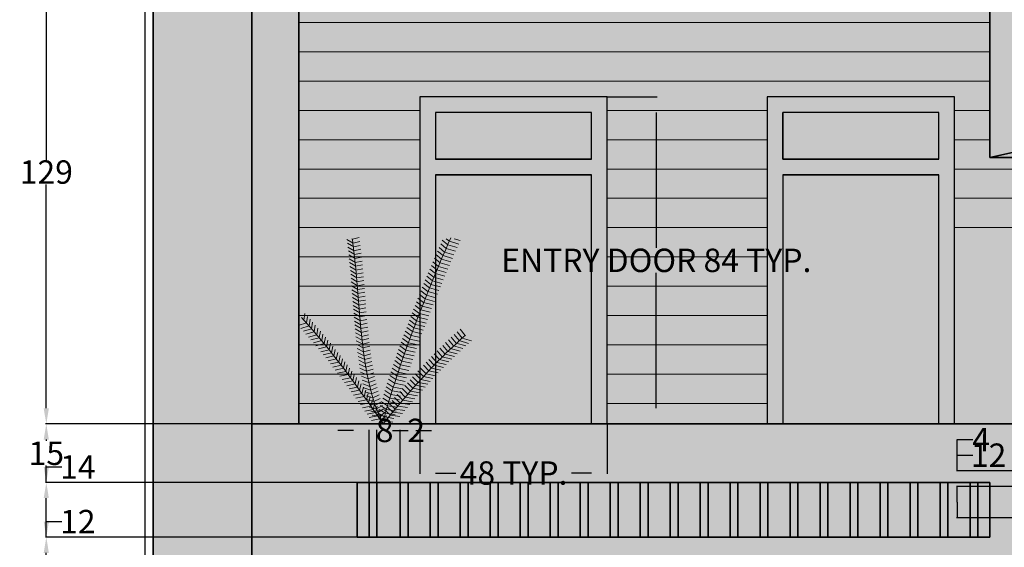
# Model space of a CAD drawing. Units: inches. Extents: x 184 to 649, y 215 to 818.
# Tile 2 of 9: x 189 to 442, y 338 to 473. Entities that reach past the tile are written whole.
import ezdxf

# ---------------------------------------------------------------- set-up
doc = ezdxf.new("R2010")
doc.units = ezdxf.units.IN
doc.header["$MEASUREMENT"] = 0
for name, color, linetype, lineweight in [('A-ANNO-DIMS', 2, 'Continuous', 18), ('A-DOOR', 4, 'Continuous', 25), ('A-ELEV', 7, 'Continuous', 35), ('A-ELEV-FILL', 9, 'Continuous', 13), ('A-ELEV-PATT', 8, 'Continuous', 13), ('L-PLNT', 84, 'Continuous', 13)]:
    doc.layers.add(name, color=color, linetype=linetype, lineweight=lineweight)
doc.styles.get("Standard").update_dxf_attribs({"font": 'arial.ttf'})
doc.dimstyles.get("Standard").update_dxf_attribs({"dimtxt": 6, "dimasz": 4, "dimexe": 0.18, "dimexo": 0.0625, "dimgap": 0.09, "dimtad": 0, "dimtih": 1, "dimtoh": 1, "dimdec": 0, "dimzin": 0, "dimdsep": 46, "dimlunit": 3, "dimtxsty": 'Standard', "dimcen": 0.09, "dimadec": 0, "dimazin": 0, "dimtfac": 1, "dimtdec": 0, "dimtofl": 0, "dimtmove": 0, "dimatfit": 3, "dimfxl": 1, "dimtolj": 1, "dimtzin": 0, "dimarcsym": 0})

# ---------------------------------------------------------------- blocks, each defined once
blk = doc.blocks.new('PLANT-PALM')
for p, q in [((274.94, 416.06), (273.31, 416.97)), ((274.8, 417.06), (274.61, 417.16)), ((274.73, 417.05), (276.46, 417.47)), ((274.87, 416.06), (276.6, 416.47)), ((299.15, 415.59), (297.73, 416.77)), ((299.55, 416.5), (298.76, 417.16)), ((299.55, 416.5), (301.94, 415.78)), ((300.78, 417.16), (302.34, 416.68)), ((275.06, 415.07), (273.44, 415.99)), ((275.18, 414.08), (273.57, 415)), ((275.3, 413.08), (273.69, 414.02)), ((275, 415.07), (276.73, 415.46)), ((275.12, 414.07), (276.85, 414.46)), ((297.95, 412.84), (296.52, 414.01)), ((298.34, 413.75), (296.92, 414.93)), ((298.74, 414.67), (297.33, 415.85)), ((298.34, 413.75), (300.74, 413.04)), ((298.74, 414.67), (301.13, 413.96)), ((299.14, 415.59), (301.53, 414.87)), ((275.4, 412.09), (273.8, 413.03)), ((275.51, 411.09), (273.9, 412.04)), ((275.23, 413.08), (276.97, 413.45)), ((275.34, 412.09), (277.08, 412.45)), ((275.44, 411.09), (277.18, 411.45)), ((296.76, 410.08), (295.33, 411.24)), ((297.16, 411), (295.73, 412.16)), ((297.55, 411.92), (296.12, 413.09)), ((297.55, 411.92), (299.94, 411.22)), ((297.94, 412.84), (300.34, 412.13)), ((275.6, 410.1), (274, 411.05)), ((275.69, 409.1), (274.1, 410.06)), ((275.78, 408.11), (274.19, 409.06)), ((275.54, 410.1), (277.28, 410.45)), ((275.63, 409.1), (277.38, 409.45)), ((295.99, 408.23), (294.55, 409.39)), ((296.38, 409.16), (294.94, 410.32)), ((296.37, 409.16), (298.78, 408.47)), ((296.76, 410.08), (299.16, 409.39)), ((297.16, 411), (299.55, 410.3)), ((275.87, 407.11), (274.28, 408.07)), ((275.95, 406.11), (274.36, 407.08)), ((275.72, 408.1), (277.47, 408.45)), ((275.81, 407.11), (277.55, 407.44)), ((275.89, 406.11), (277.64, 406.45)), ((294.84, 405.46), (293.39, 406.61)), ((295.22, 406.39), (293.78, 407.54)), ((295.6, 407.31), (294.16, 408.46)), ((295.22, 406.39), (297.62, 405.72)), ((295.6, 407.31), (298.01, 406.64)), ((295.99, 408.24), (298.39, 407.56)), ((276.03, 405.12), (274.44, 406.08)), ((276.11, 404.12), (274.52, 405.08)), ((276.19, 403.12), (274.6, 404.09)), ((275.97, 405.11), (277.72, 405.45)), ((276.05, 404.12), (277.8, 404.45)), ((293.71, 402.68), (292.26, 403.82)), ((294.08, 403.61), (292.63, 404.75)), ((294.46, 404.54), (293.01, 405.68)), ((294.08, 403.61), (296.49, 402.96)), ((294.46, 404.54), (296.87, 403.88)), ((294.84, 405.46), (297.25, 404.8)), ((276.27, 402.13), (274.68, 403.09)), ((276.35, 401.13), (274.75, 402.09)), ((276.43, 400.13), (274.83, 401.09)), ((276.13, 403.12), (277.88, 403.45)), ((276.21, 402.12), (277.96, 402.46)), ((276.29, 401.13), (278.04, 401.46)), ((292.97, 400.83), (291.51, 401.95)), ((293.34, 401.76), (291.88, 402.89)), ((293.34, 401.76), (295.75, 401.12)), ((293.71, 402.68), (296.12, 402.04)), ((276.51, 399.14), (274.91, 400.09)), ((276.59, 398.14), (274.99, 399.09)), ((276.37, 400.13), (278.12, 400.47)), ((276.45, 399.13), (278.2, 399.47)), ((291.87, 398.03), (290.41, 399.15)), ((292.24, 398.97), (290.77, 400.08)), ((292.6, 399.9), (291.14, 401.02)), ((292.24, 398.97), (294.65, 398.35)), ((292.6, 399.9), (295.02, 399.27)), ((292.97, 400.83), (295.38, 400.2)), ((262.25, 396.34), (262.49, 398.02)), ((262.93, 395.6), (263.18, 397.28)), ((263.6, 394.85), (263.86, 396.53)), ((276.67, 397.14), (275.07, 398.09)), ((276.76, 396.15), (275.15, 397.08)), ((276.84, 395.15), (275.23, 396.08)), ((276.53, 398.14), (278.28, 398.48)), ((276.62, 397.14), (278.36, 397.49)), ((276.7, 396.14), (278.45, 396.5)), ((290.8, 395.23), (289.33, 396.34)), ((291.16, 396.17), (289.68, 397.27)), ((291.51, 397.1), (290.04, 398.21)), ((291.16, 396.17), (293.58, 395.57)), ((291.51, 397.1), (293.94, 396.5)), ((291.87, 398.03), (294.29, 397.42)), ((262.93, 395.59), (260.85, 394.94)), ((263.6, 394.85), (261.51, 394.21)), ((264.26, 394.1), (262.17, 393.48)), ((264.26, 394.11), (264.53, 395.78)), ((264.91, 393.35), (265.2, 395.02)), ((265.57, 392.59), (265.86, 394.26)), ((266.21, 391.83), (266.52, 393.5)), ((276.94, 394.16), (275.32, 395.08)), ((277.03, 393.16), (275.41, 394.07)), ((276.79, 395.15), (278.54, 395.51)), ((276.89, 394.15), (278.63, 394.52)), ((276.99, 393.16), (278.72, 393.54)), ((289.75, 392.42), (288.27, 393.51)), ((290.1, 393.36), (288.62, 394.45)), ((290.45, 394.3), (288.97, 395.4)), ((290.45, 394.3), (292.88, 393.71)), ((290.8, 395.23), (293.23, 394.64)), ((303.57, 392.39), (302.33, 393.98)), ((264.92, 393.35), (262.82, 392.74)), ((265.57, 392.59), (263.47, 391.99)), ((266.22, 391.82), (264.11, 391.25)), ((266.86, 391.06), (264.75, 390.49)), ((266.85, 391.06), (267.17, 392.73)), ((267.49, 390.29), (267.81, 391.95)), ((268.12, 389.51), (268.45, 391.17)), ((277.13, 392.17), (275.5, 393.07)), ((277.24, 391.17), (275.6, 392.06)), ((277.35, 390.18), (275.71, 391.05)), ((277.09, 392.16), (278.82, 392.55)), ((277.19, 391.17), (278.93, 391.57)), ((289.07, 390.54), (287.57, 391.62)), ((289.41, 391.48), (287.92, 392.57)), ((289.41, 391.48), (291.84, 390.92)), ((289.75, 392.42), (292.18, 391.85)), ((290.1, 393.36), (292.53, 392.78)), ((300.61, 389.7), (299.32, 391.25)), ((301.34, 390.38), (300.06, 391.94)), ((302.08, 391.06), (300.81, 392.62)), ((302.82, 391.73), (301.57, 393.3)), ((302.08, 391.06), (304.47, 390.35)), ((302.82, 391.73), (305.21, 391)), ((267.49, 390.29), (265.38, 389.73)), ((268.12, 389.51), (266.01, 388.97)), ((268.75, 388.73), (266.64, 388.2)), ((268.75, 388.73), (269.09, 390.39)), ((269.37, 387.95), (269.72, 389.61)), ((269.99, 387.16), (270.34, 388.82)), ((277.47, 389.19), (275.82, 390.05)), ((277.6, 388.2), (275.94, 389.04)), ((277.31, 390.18), (279.04, 390.59)), ((277.43, 389.18), (279.15, 389.61)), ((277.56, 388.19), (279.28, 388.63)), ((288.06, 387.72), (286.56, 388.79)), ((288.39, 388.66), (286.89, 389.73)), ((288.73, 389.6), (287.23, 390.68)), ((288.39, 388.66), (290.83, 388.12)), ((288.73, 389.6), (291.16, 389.05)), ((289.07, 390.54), (291.5, 389.98)), ((298.45, 387.62), (297.13, 389.14)), ((299.16, 388.32), (297.85, 389.85)), ((299.88, 389.01), (298.59, 390.55)), ((299.88, 389.01), (302.29, 388.36)), ((300.61, 389.7), (303.01, 389.03)), ((301.34, 390.38), (303.74, 389.69)), ((269.37, 387.95), (267.26, 387.43)), ((269.99, 387.16), (267.87, 386.65)), ((270.61, 386.37), (268.48, 385.87)), ((270.6, 386.37), (270.97, 388.03)), ((271.21, 385.58), (271.58, 387.24)), ((271.82, 384.79), (272.2, 386.44)), ((277.73, 387.21), (276.06, 388.03)), ((277.87, 386.22), (276.2, 387.03)), ((278.02, 385.23), (276.34, 386.02)), ((277.69, 387.2), (279.41, 387.66)), ((277.83, 386.21), (279.55, 386.69)), ((287.08, 384.88), (285.56, 385.94)), ((287.4, 385.83), (285.89, 386.89)), ((287.73, 386.77), (286.22, 387.84)), ((287.73, 386.77), (290.17, 386.25)), ((288.06, 387.72), (290.5, 387.18)), ((295.64, 384.77), (294.28, 386.26)), ((296.33, 385.49), (294.99, 386.98)), ((297.03, 386.2), (295.69, 387.71)), ((297.74, 386.91), (296.41, 388.42)), ((297.03, 386.2), (299.46, 385.61)), ((297.74, 386.91), (300.16, 386.31)), ((298.45, 387.62), (300.87, 387)), ((299.16, 388.32), (301.58, 387.68)), ((271.22, 385.58), (269.09, 385.09)), ((271.82, 384.79), (269.7, 384.3)), ((272.43, 383.99), (270.3, 383.51)), ((272.42, 383.99), (272.8, 385.64)), ((273.02, 383.19), (273.41, 384.84)), ((273.62, 382.39), (274.01, 384.04)), ((278.18, 384.24), (276.49, 385.01)), ((278.36, 383.26), (276.65, 384)), ((277.99, 385.22), (279.69, 385.72)), ((278.15, 384.24), (279.85, 384.75)), ((278.32, 383.25), (280.02, 383.79)), ((286.44, 382.99), (284.92, 384.03)), ((286.76, 383.94), (285.24, 384.98)), ((286.75, 383.94), (289.2, 383.43)), ((287.08, 384.88), (289.52, 384.37)), ((287.4, 385.83), (289.84, 385.31)), ((293.58, 382.59), (292.2, 384.05)), ((294.26, 383.32), (292.89, 384.79)), ((294.95, 384.05), (293.58, 385.53)), ((294.95, 384.05), (297.38, 383.5)), ((295.64, 384.77), (298.07, 384.21)), ((296.33, 385.49), (298.76, 384.92)), ((273.03, 383.19), (270.9, 382.72)), ((273.62, 382.39), (271.49, 381.93)), ((274.22, 381.58), (272.09, 381.13)), ((274.21, 381.58), (274.61, 383.23)), ((274.8, 380.78), (275.21, 382.42)), ((275.39, 379.97), (275.8, 381.61)), ((278.54, 382.28), (276.83, 382.99)), ((278.74, 381.3), (277.01, 381.99)), ((278.95, 380.32), (277.21, 380.98)), ((278.51, 382.27), (280.2, 382.83)), ((278.71, 381.29), (280.39, 381.87)), ((278.92, 380.31), (280.59, 380.92)), ((285.5, 380.14), (283.97, 381.16)), ((285.81, 381.09), (284.28, 382.12)), ((286.12, 382.04), (284.6, 383.08)), ((285.81, 381.09), (288.26, 380.61)), ((286.12, 382.04), (288.57, 381.55)), ((286.44, 382.99), (288.88, 382.49)), ((290.9, 379.63), (289.48, 381.06)), ((291.56, 380.37), (290.15, 381.81)), ((292.23, 381.11), (290.83, 382.56)), ((292.9, 381.85), (291.51, 383.31)), ((292.23, 381.11), (294.68, 380.62)), ((292.9, 381.85), (295.35, 381.35)), ((293.58, 382.59), (296.02, 382.07)), ((294.26, 383.32), (296.7, 382.79)), ((274.81, 380.78), (272.68, 380.33)), ((275.4, 379.97), (273.26, 379.53)), ((275.99, 379.16), (273.85, 378.72)), ((275.98, 379.16), (276.39, 380.8)), ((276.56, 378.35), (276.98, 379.99)), ((277.14, 377.53), (277.56, 379.18)), ((279.17, 379.35), (277.42, 379.97)), ((279.41, 378.38), (277.65, 378.97)), ((277.72, 376.72), (278.15, 378.36)), ((279.15, 379.34), (280.81, 379.98)), ((279.39, 378.37), (281.04, 379.04)), ((284.9, 378.23), (283.36, 379.24)), ((285.2, 379.18), (283.66, 380.2)), ((285.2, 379.18), (287.65, 378.72)), ((285.5, 380.14), (287.95, 379.67)), ((288.92, 377.36), (287.49, 378.78)), ((289.58, 378.12), (288.15, 379.54)), ((290.23, 378.87), (288.81, 380.3)), ((290.23, 378.87), (292.69, 378.42)), ((290.9, 379.63), (293.35, 379.16)), ((291.56, 380.37), (294.01, 379.89)), ((276.57, 378.35), (274.43, 377.92)), ((277.15, 377.53), (275.02, 377.11)), ((277.74, 376.72), (275.6, 376.3)), ((278.31, 375.91), (276.18, 375.49)), ((279.67, 377.41), (277.9, 377.96)), ((279.95, 376.45), (278.16, 376.96)), ((278.3, 375.9), (278.73, 377.55)), ((280.24, 375.49), (278.44, 375.96)), ((278.88, 375.09), (279.31, 376.73)), ((279.46, 374.27), (279.88, 375.91)), ((279.65, 377.4), (281.29, 378.11)), ((279.93, 376.44), (281.55, 377.18)), ((280.23, 375.49), (281.83, 376.27)), ((284.02, 375.36), (282.47, 376.36)), ((284.31, 376.32), (282.76, 377.32)), ((284.6, 377.27), (283.06, 378.28)), ((284.31, 376.32), (286.77, 375.89)), ((284.6, 377.28), (287.06, 376.83)), ((284.9, 378.23), (287.35, 377.78)), ((286.98, 375.08), (285.53, 376.47)), ((287.63, 375.84), (286.18, 377.24)), ((288.27, 376.61), (286.83, 378.01)), ((287.63, 375.84), (290.09, 375.43)), ((288.27, 376.61), (290.73, 376.18)), ((288.92, 377.36), (291.38, 376.93)), ((289.58, 378.12), (292.03, 377.67)), ((278.89, 375.09), (276.75, 374.67)), ((279.47, 374.27), (277.33, 373.86)), ((280.05, 373.46), (277.91, 373.04)), ((280.56, 374.55), (278.75, 374.97)), ((280.9, 373.61), (279.08, 373.97)), ((280.03, 373.45), (280.46, 375.09)), ((280.55, 374.54), (282.13, 375.36)), ((280.61, 372.64), (281.04, 374.28)), ((280.89, 373.6), (282.45, 374.46)), ((281.18, 371.82), (281.61, 373.46)), ((281.26, 372.67), (282.79, 373.58)), ((283.18, 372.48), (281.61, 373.46)), ((283.45, 373.44), (281.89, 374.43)), ((283.73, 374.4), (282.18, 375.39)), ((284.44, 371.99), (282.97, 373.36)), ((283.45, 373.44), (285.92, 373.04)), ((285.07, 372.76), (283.61, 374.14)), ((283.73, 374.4), (286.2, 373.99)), ((284.02, 375.36), (286.48, 374.94)), ((285.71, 373.54), (284.24, 374.92)), ((286.34, 374.31), (284.89, 375.7)), ((285.71, 373.54), (288.17, 373.15)), ((286.34, 374.31), (288.81, 373.91)), ((286.98, 375.08), (289.45, 374.67)), ((280.62, 372.64), (278.48, 372.23)), ((281.2, 371.82), (279.05, 371.41)), ((281.26, 372.67), (279.43, 372.98)), ((281.77, 371), (279.63, 370.59)), ((281.65, 371.75), (279.81, 372)), ((282.9, 371.52), (281.33, 372.49)), ((281.65, 371.75), (283.15, 372.7)), ((281.77, 371), (282.24, 372.12)), ((282.07, 370.84), (283.54, 371.85)), ((282.9, 371.52), (285.37, 371.14)), ((283.18, 372.48), (285.64, 372.09)), ((284.44, 371.99), (286.91, 371.62)), ((285.07, 372.76), (287.54, 372.39)), ((282.63, 370.56), (285.1, 370.19))]:
    blk.add_line(p, q)
blk.add_open_spline([(274.68, 417.16), (274.77, 416.57), (276.95, 400.47), (276.36, 381.5), (282.64, 369.73)], degree=3, knots=[87.299959, 87.299959, 87.299959, 87.299959, 88.780677, 127.704389, 127.704389, 127.704389, 127.704389])
for points in [[(282.63, 370.56), (286.61, 384.99), (292.84, 401.43), (299.95, 417.41)], [(282.55, 369.88), (275.93, 379.33), (269.31, 388.78), (261.65, 396.98)], [(282.64, 369.73), (290.67, 379.89), (297.61, 387.15), (303.65, 392.43)]]:
    blk.add_open_spline(points, degree=3)
blk = doc.blocks.new('DOOR-ENTRY')
for points in [[(340, 369.73), (340, 453.5), (292, 453.5), (292, 369.73)], [(336, 437.5), (336, 449.5), (296, 449.5), (296, 437.5)], [(296, 433.5), (296, 369.73)], [(336, 369.73), (336, 433.5)]]:
    blk.add_lwpolyline(points)
blk = doc.blocks.new('*D5')
at = {"layer": 'A-ANNO-DIMS', "color": 0, "lineweight": -2, "transparency": 16777216}
for p, q in [((340.06, 453.5), (352.75, 453.5)), ((352.57, 449.5), (352.57, 414.81)), ((352.57, 373.73), (352.57, 408.42)), ((340.06, 369.73), (352.75, 369.73))]:
    blk.add_line(p, q, dxfattribs=at)
at = {"layer": 'A-ANNO-DIMS', "color": 0, "transparency": 16777216}
for points in [[(351.9, 449.5), (353.23, 449.5), (352.57, 453.5)], [(351.9, 373.73), (353.23, 373.73), (352.57, 369.73)]]:
    blk.add_solid(points, dxfattribs=at)
at = {"layer": 'Defpoints', "color": 0, "transparency": 16777216}
for p in [(340, 453.5), (352.57, 453.5), (340, 369.73)]:
    blk.add_point(p, dxfattribs=at)
at = {"layer": 'A-ANNO-DIMS', "color": 0, "transparency": 16777216, "insert": (352.57, 411.62), "char_height": 6, "attachment_point": 5}
blk.add_mtext('\\A1;ENTRY DOOR 84 TYP.', dxfattribs=at)
blk = doc.blocks.new('*D6')
at = {"layer": 'A-ANNO-DIMS', "color": 0, "lineweight": -2, "transparency": 16777216}
for p, q in [((292, 369.66), (292, 356.98)), ((340, 369.66), (340, 356.98)), ((296, 357.16), (301.19, 357.16)), ((336, 357.16), (330.81, 357.16))]:
    blk.add_line(p, q, dxfattribs=at)
at = {"layer": 'A-ANNO-DIMS', "color": 0, "transparency": 16777216}
for points in [[(296, 357.83), (296, 356.49), (292, 357.16)], [(336, 357.83), (336, 356.49), (340, 357.16)]]:
    blk.add_solid(points, dxfattribs=at)
at = {"layer": 'Defpoints', "color": 0, "transparency": 16777216}
for p in [(292, 369.73), (340, 369.73), (340, 357.16)]:
    blk.add_point(p, dxfattribs=at)
at = {"layer": 'A-ANNO-DIMS', "color": 0, "transparency": 16777216, "insert": (316, 357.16), "char_height": 6, "attachment_point": 5}
blk.add_mtext('\\A1;48 TYP.', dxfattribs=at)
blk = doc.blocks.new('*D10')
at = {"layer": 'A-ANNO-DIMS', "color": 0, "lineweight": -2, "transparency": 16777216}
for p, q in [((248.91, 786.73), (221.44, 786.73)), ((221.62, 782.73), (221.62, 519.88)), ((221.62, 250.73), (221.62, 513.57)), ((248.91, 246.73), (221.44, 246.73))]:
    blk.add_line(p, q, dxfattribs=at)
at = {"layer": 'A-ANNO-DIMS', "color": 0, "transparency": 16777216}
for points in [[(220.96, 782.73), (222.29, 782.73), (221.62, 786.73)], [(220.96, 250.73), (222.29, 250.73), (221.62, 246.73)]]:
    blk.add_solid(points, dxfattribs=at)
at = {"layer": 'Defpoints', "color": 0, "transparency": 16777216}
for p in [(221.62, 786.73), (248.97, 786.73), (248.97, 246.73)]:
    blk.add_point(p, dxfattribs=at)
at = {"layer": 'A-ANNO-DIMS', "color": 0, "transparency": 16777216, "insert": (221.62, 516.73), "char_height": 6, "attachment_point": 5}
blk.add_mtext('\\A1;540', dxfattribs=at)
blk = doc.blocks.new('*D32')
at = {"layer": 'A-ANNO-DIMS', "color": 0, "lineweight": -2, "transparency": 16777216}
for p, q in [((196.3, 340.73), (196.3, 344.73)), ((196.3, 344.73), (200.3, 344.73)), ((275.91, 340.73), (196.12, 340.73)), ((196.3, 332.73), (196.3, 336.73)), ((275.91, 328.73), (196.12, 328.73))]:
    blk.add_line(p, q, dxfattribs=at)
at = {"layer": 'A-ANNO-DIMS', "color": 0, "transparency": 16777216}
for points in [[(195.63, 336.73), (196.96, 336.73), (196.3, 340.73)], [(195.63, 332.73), (196.96, 332.73), (196.3, 328.73)]]:
    blk.add_solid(points, dxfattribs=at)
at = {"layer": 'Defpoints', "color": 0, "transparency": 16777216}
for p in [(196.3, 340.73), (275.97, 340.73), (275.97, 328.73)]:
    blk.add_point(p, dxfattribs=at)
at = {"layer": 'A-ANNO-DIMS', "color": 0, "transparency": 16777216, "insert": (204.37, 344.73), "char_height": 6, "attachment_point": 5}
blk.add_mtext('\\A1;12', dxfattribs=at)
blk = doc.blocks.new('*D33')
at = {"layer": 'A-ANNO-DIMS', "color": 0, "lineweight": -2, "transparency": 16777216}
for p, q in [((196.3, 354.73), (196.3, 358.73)), ((196.3, 358.73), (200.3, 358.73)), ((275.91, 354.73), (196.12, 354.73)), ((196.3, 344.73), (196.3, 350.73)), ((275.91, 340.73), (196.12, 340.73))]:
    blk.add_line(p, q, dxfattribs=at)
at = {"layer": 'A-ANNO-DIMS', "color": 0, "transparency": 16777216}
for points in [[(195.63, 350.73), (196.96, 350.73), (196.3, 354.73)], [(195.63, 344.73), (196.96, 344.73), (196.3, 340.73)]]:
    blk.add_solid(points, dxfattribs=at)
at = {"layer": 'Defpoints', "color": 0, "transparency": 16777216}
for p in [(196.3, 354.73), (275.97, 354.73), (275.97, 340.73)]:
    blk.add_point(p, dxfattribs=at)
at = {"layer": 'A-ANNO-DIMS', "color": 0, "transparency": 16777216, "insert": (204.39, 358.73), "char_height": 6, "attachment_point": 5}
blk.add_mtext('\\A1;14', dxfattribs=at)
blk = doc.blocks.new('*D34')
at = {"layer": 'A-ANNO-DIMS', "color": 0, "lineweight": -2, "transparency": 16777216}
for p, q in [((248.91, 369.73), (196.12, 369.73)), ((196.3, 365.73), (196.3, 365.38)), ((196.3, 358.73), (196.3, 359.07)), ((275.91, 354.73), (196.12, 354.73))]:
    blk.add_line(p, q, dxfattribs=at)
at = {"layer": 'A-ANNO-DIMS', "color": 0, "transparency": 16777216}
for points in [[(195.63, 365.73), (196.96, 365.73), (196.3, 369.73)], [(195.63, 358.73), (196.96, 358.73), (196.3, 354.73)]]:
    blk.add_solid(points, dxfattribs=at)
at = {"layer": 'Defpoints', "color": 0, "transparency": 16777216}
for p in [(196.3, 369.73), (248.97, 369.73), (275.97, 354.73)]:
    blk.add_point(p, dxfattribs=at)
at = {"layer": 'A-ANNO-DIMS', "color": 0, "transparency": 16777216, "insert": (196.3, 362.23), "char_height": 6, "attachment_point": 5}
blk.add_mtext('\\A1;15', dxfattribs=at)
blk = doc.blocks.new('*D35')
at = {"layer": 'A-ANNO-DIMS', "color": 0, "lineweight": -2, "transparency": 16777216}
for p, q in [((260.91, 498.73), (196.12, 498.73)), ((196.3, 494.73), (196.3, 437.38)), ((196.3, 373.73), (196.3, 431.07)), ((260.91, 369.73), (196.12, 369.73))]:
    blk.add_line(p, q, dxfattribs=at)
at = {"layer": 'A-ANNO-DIMS', "color": 0, "transparency": 16777216}
for points in [[(195.63, 494.73), (196.96, 494.73), (196.3, 498.73)], [(195.63, 373.73), (196.96, 373.73), (196.3, 369.73)]]:
    blk.add_solid(points, dxfattribs=at)
at = {"layer": 'Defpoints', "color": 0, "transparency": 16777216}
for p in [(196.3, 498.73), (260.97, 498.73), (260.97, 369.73)]:
    blk.add_point(p, dxfattribs=at)
at = {"layer": 'A-ANNO-DIMS', "color": 0, "transparency": 16777216, "insert": (196.3, 434.23), "char_height": 6, "attachment_point": 5}
blk.add_mtext('\\A1;129', dxfattribs=at)
blk = doc.blocks.new('*D68')
at = {"layer": 'A-ANNO-DIMS', "color": 0, "lineweight": -2, "transparency": 16777216}
for p, q in [((274.97, 368.08), (270.97, 368.08)), ((278.97, 340.79), (278.97, 368.26)), ((280.97, 340.79), (280.97, 368.26)), ((284.97, 368.08), (288.97, 368.08))]:
    blk.add_line(p, q, dxfattribs=at)
at = {"layer": 'A-ANNO-DIMS', "color": 0, "transparency": 16777216}
for points in [[(274.97, 368.74), (274.97, 367.41), (278.97, 368.08)], [(284.97, 368.74), (284.97, 367.41), (280.97, 368.08)]]:
    blk.add_solid(points, dxfattribs=at)
at = {"layer": 'Defpoints', "color": 0, "transparency": 16777216}
for p in [(280.97, 368.08), (278.97, 340.73), (280.97, 340.73)]:
    blk.add_point(p, dxfattribs=at)
at = {"layer": 'A-ANNO-DIMS', "color": 0, "transparency": 16777216, "insert": (291.05, 368.08), "char_height": 6, "attachment_point": 5}
blk.add_mtext('\\A1;2', dxfattribs=at)
blk = doc.blocks.new('*D69')
at = {"layer": 'A-ANNO-DIMS', "color": 0, "lineweight": -2, "transparency": 16777216}
for p, q in [((274.97, 368.08), (270.97, 368.08)), ((278.97, 340.79), (278.97, 368.26)), ((286.97, 340.79), (286.97, 368.26)), ((290.97, 368.08), (294.97, 368.08))]:
    blk.add_line(p, q, dxfattribs=at)
at = {"layer": 'A-ANNO-DIMS', "color": 0, "transparency": 16777216}
for points in [[(274.97, 368.74), (274.97, 367.41), (278.97, 368.08)], [(290.97, 368.74), (290.97, 367.41), (286.97, 368.08)]]:
    blk.add_solid(points, dxfattribs=at)
at = {"layer": 'Defpoints', "color": 0, "transparency": 16777216}
for p in [(286.97, 368.08), (278.97, 340.73), (286.97, 340.73)]:
    blk.add_point(p, dxfattribs=at)
at = {"layer": 'A-ANNO-DIMS', "color": 0, "transparency": 16777216, "insert": (282.97, 368.08), "char_height": 6, "attachment_point": 5}
blk.add_mtext('\\A1;8', dxfattribs=at)
blk = doc.blocks.new('*D71')
at = {"layer": 'A-ANNO-DIMS', "color": 0, "lineweight": -2, "transparency": 16777216}
for p, q in [((429.62, 361.73), (429.62, 365.73)), ((429.62, 365.73), (433.62, 365.73)), ((456.91, 357.73), (429.44, 357.73)), ((456.91, 353.73), (429.44, 353.73)), ((429.62, 349.73), (429.62, 345.73))]:
    blk.add_line(p, q, dxfattribs=at)
at = {"layer": 'A-ANNO-DIMS', "color": 0, "transparency": 16777216}
for points in [[(428.96, 361.73), (430.29, 361.73), (429.62, 357.73)], [(428.96, 349.73), (430.29, 349.73), (429.62, 353.73)]]:
    blk.add_solid(points, dxfattribs=at)
at = {"layer": 'Defpoints', "color": 0, "transparency": 16777216}
for p in [(429.62, 357.73), (456.97, 357.73), (456.97, 353.73)]:
    blk.add_point(p, dxfattribs=at)
at = {"layer": 'A-ANNO-DIMS', "color": 0, "transparency": 16777216, "insert": (435.79, 365.73), "char_height": 6, "attachment_point": 5}
blk.add_mtext('\\A1;4', dxfattribs=at)
blk = doc.blocks.new('*D72')
at = {"layer": 'A-ANNO-DIMS', "color": 0, "lineweight": -2, "transparency": 16777216}
for p, q in [((429.62, 357.73), (429.62, 361.73)), ((429.62, 361.73), (433.62, 361.73)), ((456.91, 357.73), (429.44, 357.73)), ((429.62, 349.73), (429.62, 353.73)), ((456.91, 345.73), (429.44, 345.73))]:
    blk.add_line(p, q, dxfattribs=at)
at = {"layer": 'A-ANNO-DIMS', "color": 0, "transparency": 16777216}
for points in [[(428.96, 353.73), (430.29, 353.73), (429.62, 357.73)], [(428.96, 349.73), (430.29, 349.73), (429.62, 345.73)]]:
    blk.add_solid(points, dxfattribs=at)
at = {"layer": 'Defpoints', "color": 0, "transparency": 16777216}
for p in [(429.62, 357.73), (456.97, 357.73), (456.97, 345.73)]:
    blk.add_point(p, dxfattribs=at)
at = {"layer": 'A-ANNO-DIMS', "color": 0, "transparency": 16777216, "insert": (437.7, 361.73), "char_height": 6, "attachment_point": 5}
blk.add_mtext('\\A1;12', dxfattribs=at)

msp = doc.modelspace()

# ---------------------------------------------------------------- hatches: boundary and pattern name
at = {"layer": 'A-ELEV-FILL'}
h = msp.add_hatch(color=256, dxfattribs=at)
h.dxf.hatch_style = 1
h.paths.add_polyline_path([(248.9726, 786.7265), (223.6471, 761.141), (223.6471, 257.141), (248.9726, 246.7265)])
h = msp.add_hatch(color=256, dxfattribs=at)
h.dxf.hatch_style = 1
h.paths.add_polyline_path([(452.9726, 369.7265), (248.9726, 369.7265), (248.9726, 246.7265), (275.9726, 246.7265), (275.9726, 328.7265), (437.9726, 328.7265), (437.9726, 246.7265), (446.6666, 246.7265), (452.9726, 282.7265)])
h.paths.add_polyline_path([(275.9726, 340.7265), (275.9726, 354.7265), (437.9726, 354.7265), (437.9726, 340.7265)], flags=16)
h.paths.add_polyline_path([(452.9726, 510.7265), (260.9726, 510.7265), (260.9726, 642.7265), (260.9726, 699.7265), (367.0226, 699.7265), (373.9381, 706.7265), (260.9726, 706.7265), (260.9726, 715.7265), (382.8295, 715.7265), (389.745, 722.7265), (260.9726, 722.7265), (260.9726, 731.7265), (398.6364, 731.7265), (405.5519, 738.7265), (260.9726, 738.7265), (260.9726, 747.7265), (414.4433, 747.7265), (421.3588, 754.7265), (260.9726, 754.7265), (260.9726, 763.7265), (430.2502, 763.7265), (437.1657, 770.7265), (260.9726, 770.7265), (260.9726, 779.7265), (446.057, 779.7265), (452.9726, 786.7265), (248.9726, 786.7265), (248.9726, 369.7265), (260.9726, 369.7265), (260.9726, 498.7265), (452.9726, 498.7265)])
h = msp.add_hatch(color=256, dxfattribs=at)
h.dxf.hatch_style = 1
h.paths.add_polyline_path([(380.9726, 453.5037), (422.2268, 453.5037), (422.2268, 474.7265), (260.9726, 474.7265), (260.9726, 369.7265), (291.9998, 369.7265), (291.9998, 453.5037), (339.9998, 453.5037), (339.9998, 369.7265), (380.9726, 369.7265)])
h.paths.add_polyline_path([(437.9726, 328.7265), (275.9726, 328.7265), (275.9726, 246.7265), (437.9726, 246.7265)])
h.paths.add_polyline_path([(581.9726, 759.7265), (521.9726, 759.7265), (521.9726, 441.2233), (581.9726, 441.2233)])
h.paths.add_polyline_path([(560.9726, 582.4749), (560.9726, 477.2233), (542.9726, 477.2233), (542.9726, 582.4749)], flags=16)
h.paths.add_polyline_path([(560.9726, 618.4749), (542.9726, 618.4749), (542.9726, 723.7265), (560.9726, 723.7265)], flags=16)
h = msp.add_hatch(color=256, dxfattribs=at)
h.dxf.hatch_style = 1
h.paths.add_polyline_path([(335.9998, 433.5037), (295.9998, 433.5037), (295.9998, 369.7265), (335.9998, 369.7265)])
h.paths.add_polyline_path([(335.9998, 449.5037), (295.9998, 449.5037), (295.9998, 437.5037), (335.9998, 437.5037)])
h.paths.add_polyline_path([(422.2268, 449.5037), (384.9726, 449.5037), (384.9726, 437.5037), (422.2268, 437.5037)])
h.paths.add_polyline_path([(422.2268, 433.5037), (384.9726, 433.5037), (384.9726, 369.7265), (422.2268, 369.7265)])
h.paths.add_polyline_path([(335.9998, 590.7265), (295.9998, 590.7265), (295.9998, 578.7265), (335.9998, 578.7265)])
h.paths.add_polyline_path([(335.9998, 574.7265), (295.9998, 574.7265), (295.9998, 548.7265), (335.9998, 548.7265)])
h.paths.add_polyline_path([(422.9726, 590.7265), (384.9726, 590.7265), (384.9726, 578.7265), (422.9726, 578.7265)])
h.paths.add_polyline_path([(422.9726, 574.7265), (384.9726, 574.7265), (384.9726, 548.7265), (422.9726, 548.7265)])
h = msp.add_hatch(color=256, dxfattribs=at)
h.dxf.hatch_style = 1
h.paths.add_polyline_path([(417.6041, 354.7265), (411.9199, 354.7265), (411.9199, 340.7265), (417.6041, 340.7265)])
h.paths.add_polyline_path([(409.9199, 354.7265), (404.2357, 354.7265), (404.2357, 340.7265), (409.9199, 340.7265)])
h.paths.add_polyline_path([(402.2357, 354.7265), (396.5515, 354.7265), (396.5515, 340.7265), (402.2357, 340.7265)])
h.paths.add_polyline_path([(394.5515, 354.7265), (388.8673, 354.7265), (388.8673, 340.7265), (394.5515, 340.7265)])
h.paths.add_polyline_path([(333.0778, 354.7265), (327.3936, 354.7265), (327.3936, 340.7265), (333.0778, 340.7265)])
h.paths.add_polyline_path([(325.3936, 354.7265), (319.7094, 354.7265), (319.7094, 340.7265), (325.3936, 340.7265)])
h.paths.add_polyline_path([(317.7094, 354.7265), (312.0252, 354.7265), (312.0252, 340.7265), (317.7094, 340.7265)])
h.paths.add_polyline_path([(310.0252, 354.7265), (304.341, 354.7265), (304.341, 340.7265), (310.0252, 340.7265)])
h.paths.add_polyline_path([(302.341, 354.7265), (296.6568, 354.7265), (296.6568, 340.7265), (302.341, 340.7265)])
h.paths.add_polyline_path([(421.3174, 546.7265), (416.9036, 546.7265), (416.9036, 514.7265), (421.3174, 514.7265)])
h.paths.add_polyline_path([(414.9036, 546.7265), (410.4898, 546.7265), (410.4898, 514.7265), (414.9036, 514.7265)])
h.paths.add_polyline_path([(402.076, 546.7265), (397.6622, 546.7265), (397.6622, 514.7265), (402.076, 514.7265)])
h.paths.add_polyline_path([(395.6622, 546.7265), (391.2484, 546.7265), (391.2484, 514.7265), (395.6622, 514.7265)])
h.paths.add_polyline_path([(389.2484, 546.7265), (384.9726, 546.7265), (384.9726, 514.7265), (389.2484, 514.7265)])
h.paths.add_polyline_path([(408.4898, 546.7265), (404.076, 546.7265), (404.076, 514.7265), (408.4898, 514.7265)])
h.paths.add_polyline_path([(335.9998, 546.7265), (333.5243, 546.7265), (333.5243, 514.7265), (335.9998, 514.7265)])
h.paths.add_polyline_path([(331.5243, 546.7265), (327.1105, 546.7265), (327.1105, 514.7265), (331.5243, 514.7265)])
h.paths.add_polyline_path([(325.1105, 546.7265), (320.6967, 546.7265), (320.6967, 514.7265), (325.1105, 514.7265)])
h.paths.add_polyline_path([(318.6967, 546.7265), (314.2829, 546.7265), (314.2829, 514.7265), (318.6967, 514.7265)])
h.paths.add_polyline_path([(312.2829, 546.7265), (307.8691, 546.7265), (307.8691, 514.7265), (312.2829, 514.7265)])
h.paths.add_polyline_path([(305.8691, 546.7265), (301.4553, 546.7265), (301.4553, 514.7265), (305.8691, 514.7265)])
h.paths.add_polyline_path([(299.4553, 546.7265), (295.9998, 546.7265), (295.9998, 514.7265), (299.4553, 514.7265)])
h = msp.add_hatch(color=256, dxfattribs=at)
h.dxf.hatch_style = 1
h.paths.add_polyline_path([(437.9726, 498.7265), (260.9726, 498.7265), (260.9726, 474.7265), (422.2268, 474.7265), (422.2268, 453.5037), (428.9726, 453.5037), (428.9726, 417.0753), (445.4726, 417.0753), (445.4726, 437.9607), (437.9726, 437.9607)])
h = msp.add_hatch(color=256, dxfattribs=at)
h.dxf.hatch_style = 1
h.paths.add_polyline_path([(452.9726, 498.7265), (437.9726, 498.7265), (437.9726, 437.9607), (452.9726, 441.2233)])
h = msp.add_hatch(color=256, dxfattribs=at)
h.dxf.hatch_style = 1
h.paths.add_polyline_path([(339.9998, 453.5037), (291.9998, 453.5037), (291.9998, 369.7265), (295.9998, 369.7265), (295.9998, 433.5037), (335.9998, 433.5037), (335.9998, 369.7265), (339.9998, 369.7265)])
h.paths.add_polyline_path([(295.9998, 449.5037), (335.9998, 449.5037), (335.9998, 437.5037), (295.9998, 437.5037)], flags=16)
h.paths.add_polyline_path([(422.2268, 453.5037), (380.9726, 453.5037), (380.9726, 369.7265), (384.9726, 369.7265), (384.9726, 433.5037), (422.2268, 433.5037), (422.2268, 437.5037), (384.9726, 437.5037), (384.9726, 449.5037), (422.2268, 449.5037)])
h = msp.add_hatch(color=256, dxfattribs=at)
h.dxf.hatch_style = 1
h.paths.add_polyline_path([(428.9726, 453.5037), (422.2268, 453.5037), (422.2268, 449.5037), (424.9726, 449.5037), (424.9726, 437.5037), (422.2268, 437.5037), (422.2268, 433.5037), (424.9726, 433.5037), (424.9726, 417.0753), (428.9726, 417.0753)])
h = msp.add_hatch(color=256, dxfattribs=at)
h.dxf.hatch_style = 1
h.paths.add_polyline_path([(424.9726, 433.5037), (422.2268, 433.5037), (422.2268, 417.0753), (424.9726, 417.0753)])
h.paths.add_polyline_path([(424.9726, 449.5037), (422.2268, 449.5037), (422.2268, 437.5037), (424.9726, 437.5037)])
h = msp.add_hatch(color=256, dxfattribs=at)
h.dxf.hatch_style = 1
h.paths.add_polyline_path([(581.9726, 441.2233), (452.9726, 441.2233), (437.9726, 437.9607), (581.9726, 437.9607)])
h = msp.add_hatch(color=256, dxfattribs=at)
h.dxf.hatch_style = 1
h.paths.add_polyline_path([(424.9726, 417.0753), (422.2268, 417.0753), (422.2268, 433.5037), (384.9726, 433.5037), (384.9726, 369.7265), (424.9726, 369.7265)])
h = msp.add_hatch(color=256, dxfattribs=at)
h.dxf.hatch_style = 1
h.paths.add_polyline_path([(428.9726, 417.0753), (424.9726, 417.0753), (424.9726, 369.7265), (428.9726, 369.7265)])
h = msp.add_hatch(color=256, dxfattribs=at)
h.dxf.hatch_style = 1
h.paths.add_polyline_path([(445.4726, 417.0753), (428.9726, 417.0753), (428.9726, 369.7265), (445.4726, 369.7265)])
h = msp.add_hatch(color=256, dxfattribs=at)
h.dxf.hatch_style = 1
h.paths.add_polyline_path([(286.9726, 354.7265), (280.9726, 354.7265), (280.9726, 340.7265), (286.9726, 340.7265)])
h.paths.add_polyline_path([(278.9726, 354.7265), (275.9726, 354.7265), (275.9726, 340.7265), (278.9726, 340.7265)])
h.paths.add_polyline_path([(294.6568, 354.7265), (288.9726, 354.7265), (288.9726, 340.7265), (294.6568, 340.7265)])
h.paths.add_polyline_path([(348.4462, 354.7265), (342.762, 354.7265), (342.762, 340.7265), (348.4462, 340.7265)])
h.paths.add_polyline_path([(356.1305, 354.7265), (350.4462, 354.7265), (350.4462, 340.7265), (356.1305, 340.7265)])
h.paths.add_polyline_path([(363.8147, 354.7265), (358.1305, 354.7265), (358.1305, 340.7265), (363.8147, 340.7265)])
h.paths.add_polyline_path([(371.4989, 354.7265), (365.8147, 354.7265), (365.8147, 340.7265), (371.4989, 340.7265)])
h.paths.add_polyline_path([(379.1831, 354.7265), (373.4989, 354.7265), (373.4989, 340.7265), (379.1831, 340.7265)])
h.paths.add_polyline_path([(432.9726, 354.7265), (427.2883, 354.7265), (427.2883, 340.7265), (432.9726, 340.7265)])
h.paths.add_polyline_path([(437.9726, 354.7265), (434.9726, 354.7265), (434.9726, 340.7265), (437.9726, 340.7265)])
h = msp.add_hatch(color=256, dxfattribs=at)
h.dxf.hatch_style = 1
h.paths.add_polyline_path([(280.9726, 354.7265), (278.9726, 354.7265), (278.9726, 340.7265), (280.9726, 340.7265)])
h.paths.add_polyline_path([(288.9726, 354.7265), (286.9726, 354.7265), (286.9726, 340.7265), (288.9726, 340.7265)])
h.paths.add_polyline_path([(296.6568, 354.7265), (294.6568, 354.7265), (294.6568, 340.7265), (296.6568, 340.7265)])
h.paths.add_polyline_path([(304.341, 354.7265), (302.341, 354.7265), (302.341, 340.7265), (304.341, 340.7265)])
h.paths.add_polyline_path([(312.0252, 354.7265), (310.0252, 354.7265), (310.0252, 340.7265), (312.0252, 340.7265)])
h.paths.add_polyline_path([(319.7094, 354.7265), (317.7094, 354.7265), (317.7094, 340.7265), (319.7094, 340.7265)])
h.paths.add_polyline_path([(327.3936, 354.7265), (325.3936, 354.7265), (325.3936, 340.7265), (327.3936, 340.7265)])
h.paths.add_polyline_path([(335.0778, 354.7265), (333.0778, 354.7265), (333.0778, 340.7265), (335.0778, 340.7265)])
h.paths.add_polyline_path([(342.762, 354.7265), (340.762, 354.7265), (340.762, 340.7265), (342.762, 340.7265)])
h.paths.add_polyline_path([(350.4462, 354.7265), (348.4462, 354.7265), (348.4462, 340.7265), (350.4462, 340.7265)])
h.paths.add_polyline_path([(358.1305, 354.7265), (356.1305, 354.7265), (356.1305, 340.7265), (358.1305, 340.7265)])
h.paths.add_polyline_path([(365.8147, 354.7265), (363.8147, 354.7265), (363.8147, 340.7265), (365.8147, 340.7265)])
h.paths.add_polyline_path([(373.4989, 354.7265), (371.4989, 354.7265), (371.4989, 340.7265), (373.4989, 340.7265)])
h.paths.add_polyline_path([(381.1831, 354.7265), (379.1831, 354.7265), (379.1831, 340.7265), (381.1831, 340.7265)])
h.paths.add_polyline_path([(388.8673, 354.7265), (386.8673, 354.7265), (386.8673, 340.7265), (388.8673, 340.7265)])
h.paths.add_polyline_path([(396.5515, 354.7265), (394.5515, 354.7265), (394.5515, 340.7265), (396.5515, 340.7265)])
h.paths.add_polyline_path([(404.2357, 354.7265), (402.2357, 354.7265), (402.2357, 340.7265), (404.2357, 340.7265)])
h.paths.add_polyline_path([(411.9199, 354.7265), (409.9199, 354.7265), (409.9199, 340.7265), (411.9199, 340.7265)])
h.paths.add_polyline_path([(419.6041, 354.7265), (417.6041, 354.7265), (417.6041, 340.7265), (419.6041, 340.7265)])
h.paths.add_polyline_path([(427.2883, 354.7265), (425.2883, 354.7265), (425.2883, 340.7265), (427.2883, 340.7265)])
h.paths.add_polyline_path([(434.9726, 354.7265), (432.9726, 354.7265), (432.9726, 340.7265), (434.9726, 340.7265)])
h = msp.add_hatch(color=256, dxfattribs=at)
h.dxf.hatch_style = 1
h.paths.add_polyline_path([(340.762, 354.7265), (335.0778, 354.7265), (335.0778, 340.7265), (340.762, 340.7265)])
h.paths.add_polyline_path([(386.8673, 354.7265), (381.1831, 354.7265), (381.1831, 340.7265), (386.8673, 340.7265)])
h.paths.add_polyline_path([(425.2883, 354.7265), (419.6041, 354.7265), (419.6041, 340.7265), (425.2883, 340.7265)])
at = {"layer": 'A-ELEV-PATT'}
h = msp.add_hatch(dxfattribs=at)
h.set_pattern_fill('ANSI31', color=256, scale=60, angle=135)
h.paths.add_polyline_path([(437.9726, 498.7265), (260.9726, 498.7265), (260.9726, 369.7265), (291.9998, 369.7265), (291.9998, 453.5037), (339.9998, 453.5037), (339.9998, 369.7265), (380.9726, 369.7265), (380.9726, 453.5037), (428.9726, 453.5037), (428.9726, 417.0753), (445.4726, 417.0753), (445.4726, 437.9607), (437.9726, 437.9607)])

# ---------------------------------------------------------------- linework, layer by layer
at = {"layer": 'A-ELEV'}
for p, q in [((248.9726, 786.7265), (248.9726, 246.7265)), ((223.6471, 761.141), (223.6471, 257.141)), ((260.9726, 498.7265), (260.9726, 369.7265)), ((437.9726, 437.9607), (437.9726, 498.7265)), ((384.9726, 449.5037), (384.9726, 437.5037)), ((452.9726, 441.2233), (437.9726, 437.9607)), ((295.9998, 437.5037), (335.9998, 437.5037)), ((384.9726, 437.5037), (424.9726, 437.5037)), ((437.9726, 437.9607), (581.9726, 437.9607)), ((335.9998, 433.5037), (295.9998, 433.5037)), ((424.9726, 433.5037), (384.9726, 433.5037)), ((596.9726, 369.7265), (248.9726, 369.7265)), ((275.9726, 354.7265), (275.9726, 340.7265)), ((437.9726, 354.7265), (275.9726, 354.7265)), ((278.9726, 354.7265), (278.9726, 340.7265)), ((280.9726, 354.7265), (280.9726, 340.7265)), ((286.9726, 354.7265), (286.9726, 340.7265)), ((288.9726, 354.7265), (288.9726, 340.7265)), ((294.6568, 354.7265), (294.6568, 340.7265)), ((296.6568, 354.7265), (296.6568, 340.7265)), ((302.341, 354.7265), (302.341, 340.7265)), ((304.341, 354.7265), (304.341, 340.7265)), ((310.0252, 354.7265), (310.0252, 340.7265)), ((312.0252, 354.7265), (312.0252, 340.7265)), ((317.7094, 354.7265), (317.7094, 340.7265)), ((319.7094, 354.7265), (319.7094, 340.7265)), ((325.3936, 354.7265), (325.3936, 340.7265)), ((327.3936, 354.7265), (327.3936, 340.7265)), ((333.0778, 354.7265), (333.0778, 340.7265)), ((335.0778, 354.7265), (335.0778, 340.7265)), ((340.762, 354.7265), (340.762, 340.7265)), ((342.762, 354.7265), (342.762, 340.7265)), ((348.4462, 354.7265), (348.4462, 340.7265)), ((350.4462, 354.7265), (350.4462, 340.7265)), ((356.1305, 354.7265), (356.1305, 340.7265)), ((358.1305, 354.7265), (358.1305, 340.7265)), ((363.8147, 354.7265), (363.8147, 340.7265)), ((365.8147, 354.7265), (365.8147, 340.7265)), ((371.4989, 354.7265), (371.4989, 340.7265)), ((373.4989, 354.7265), (373.4989, 340.7265)), ((379.1831, 354.7265), (379.1831, 340.7265)), ((381.1831, 354.7265), (381.1831, 340.7265)), ((386.8673, 354.7265), (386.8673, 340.7265)), ((388.8673, 354.7265), (388.8673, 340.7265)), ((394.5515, 354.7265), (394.5515, 340.7265)), ((396.5515, 354.7265), (396.5515, 340.7265)), ((402.2357, 354.7265), (402.2357, 340.7265)), ((404.2357, 354.7265), (404.2357, 340.7265)), ((409.9199, 354.7265), (409.9199, 340.7265)), ((411.9199, 354.7265), (411.9199, 340.7265)), ((417.6041, 354.7265), (417.6041, 340.7265)), ((419.6041, 354.7265), (419.6041, 340.7265)), ((425.2883, 354.7265), (425.2883, 340.7265)), ((427.2883, 354.7265), (427.2883, 340.7265)), ((432.9726, 354.7265), (432.9726, 340.7265)), ((434.9726, 354.7265), (434.9726, 340.7265)), ((437.9726, 340.7265), (437.9726, 354.7265)), ((437.9726, 340.7265), (275.9726, 340.7265))]:
    msp.add_line(p, q, dxfattribs=at)

# ---------------------------------------------------------------- block references
at = {"layer": 'A-DOOR'}
for p in [(0, 0), (88.9728, 0)]:
    msp.add_blockref('DOOR-ENTRY', p, dxfattribs=at)
at = {"layer": 'L-PLNT'}
msp.add_blockref('PLANT-PALM', (0, 0), dxfattribs=at)

# ---------------------------------------------------------------- dimensions: what is measured, and where the dimension line sits
at = {"layer": 'A-ANNO-DIMS'}
for base, p1, p2, picture, middle in [((221.6226, 786.7265), (248.9726, 246.7265), (248.9726, 786.7265), '*D10', (221.6226, 516.7265)), ((196.2971, 498.7265), (260.9726, 369.7265), (260.9726, 498.7265), '*D35', (196.2971, 434.2265)), ((196.2971, 369.7265), (275.9726, 354.7265), (248.9726, 369.7265), '*D34', (196.2971, 362.2265)), ((429.6226, 357.7265), (456.9726, 353.7265), (456.9726, 357.7265), '*D71', (435.7876, 365.7265)), ((429.6226, 357.7265), (456.9726, 345.7265), (456.9726, 357.7265), '*D72', (437.6969, 361.7265)), ((196.2971, 354.7265), (275.9726, 340.7265), (275.9726, 354.7265), '*D33', (204.3898, 358.7265)), ((196.2971, 340.7265), (275.9726, 328.7265), (275.9726, 340.7265), '*D32', (204.3714, 344.7265))]:
    dim = msp.add_linear_dim(base=base, p1=p1, p2=p2, angle=90, dimstyle='Standard', override={"dimdec": 0, "dimlfac": 1, "dimrnd": 0, "dimzin": 0, "dimdsep": 46, "dimlunit": 2}, dxfattribs=at)
    dim.commit()
    dim.dimension.update_dxf_attribs({"geometry": picture, "text_midpoint": middle})
dim = msp.add_linear_dim(base=(352.5664, 453.5037), p1=(339.9998, 369.7265), p2=(339.9998, 453.5037), angle=90, text='ENTRY DOOR <> TYP.', dimstyle='Standard', override={"dimdec": 0, "dimrnd": 0, "dimzin": 0, "dimlunit": 2}, dxfattribs=at)
dim.commit()
dim.dimension.update_dxf_attribs({"geometry": '*D5', "text_midpoint": (352.5664, 411.6151)})
for base, p2, picture, middle in [((280.9726, 368.0765), (280.9726, 340.7265), '*D68', (291.0496, 368.0765)), ((286.9726, 368.0765), (286.9726, 340.7265), '*D69', (282.9726, 368.0765))]:
    dim = msp.add_linear_dim(base=base, p1=(278.9726, 340.7265), p2=p2, dimstyle='Standard', override={"dimdec": 0, "dimlfac": 1, "dimrnd": 0, "dimzin": 0, "dimdsep": 46, "dimlunit": 2}, dxfattribs=at)
    dim.commit()
    dim.dimension.update_dxf_attribs({"geometry": picture, "text_midpoint": middle})
dim = msp.add_linear_dim(base=(339.9998, 357.16), p1=(291.9998, 369.7265), p2=(339.9998, 369.7265), text='<> TYP.', dimstyle='Standard', override={"dimdec": 0, "dimrnd": 0, "dimzin": 0, "dimlunit": 2}, dxfattribs=at)
dim.commit()
dim.dimension.update_dxf_attribs({"geometry": '*D6', "text_midpoint": (315.9998, 357.16)})

doc.saveas('drawing.dxf')
